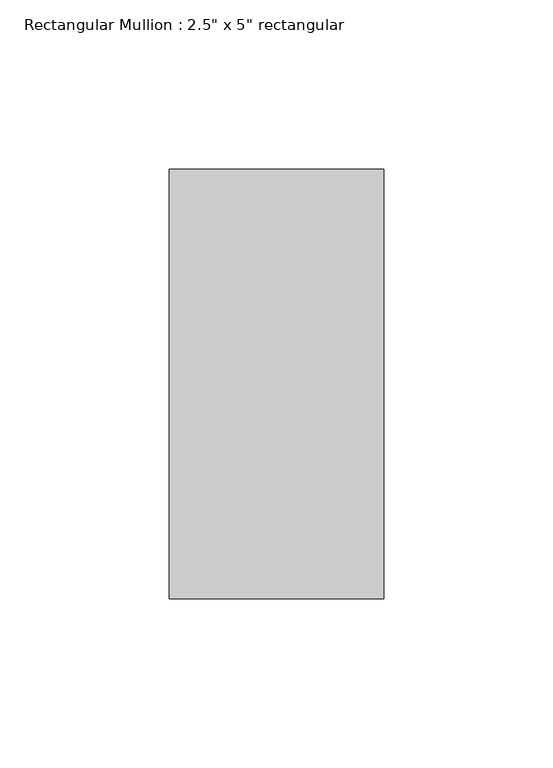
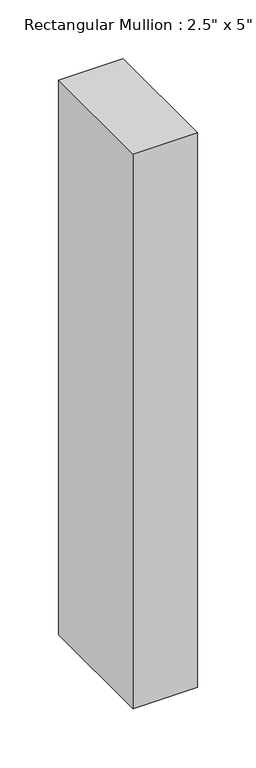
"""IFC4 building model written with IfcOpenShell, lengths in millimetres: member geometry."""

from ifc_helpers import new_model, si_unit, frame, origin, place, context, project, spatial, polyline, outline, extrude, source, transform, mapped, element, save


def member_af2dc76d(model_context):
    return source(origin(), model_context, "Body", "SweptSolid", [
        extrude(outline(polyline([(0.0, 63.5), (0.0, -63.5), (-63.5, -63.5), (-63.5, 63.5), (0.0, 63.5)])), frame((0.0, 0.0, -577.9826807), z_axis=(0.0, 0.0, 1.0), x_axis=(1.0, 0.0, 0.0)), (0.0, 0.0, 1.0), 577.9826807),
    ])


if __name__ == "__main__":
    model = new_model("IFC4")
    model_context = context("Model", 3, world=origin())
    ifc_project = project(units=[si_unit("LENGTHUNIT", "METRE", prefix="MILLI")], contexts=[model_context])
    site = spatial("IfcSite", under=ifc_project)
    building = spatial("IfcBuilding", under=site)
    placement = place(None, origin())
    member_shape = member_af2dc76d(model_context)
    element("IfcMember", 1, ObjectType="Rectangular Mullion : 2.5\" x 5\" rectangular", at=placement, inside=building, context=model_context, shape_type="MappedRepresentation", body=[
        mapped(member_shape, transform((0.0, 0.0, 0.0), x_axis=(1.0, 0.0, 0.0), y_axis=(0.0, 1.0, 0.0), z_axis=(0.0, 0.0, 1.0))),
    ])
    save(model, "model.ifc")

# Revit data of these elements
# Type "Rectangular Mullion : 2.5\" x 5\" rectangular"
#   built-in parameter 1007304 = 0.416667 (stored number, unit not read)
#   built-in parameter 1007301 = 0.104167 (stored number, unit not read)
#   built-in parameter 1007300 = 0.104167 (stored number, unit not read)
# Element 1 (IfcMember, "Rectangular Mullion : 2.5\" x 5\" rectangular")
#   Materials on its faces: "Aluminum"
# Materials
#   "Aluminum": class "Metal", colour RGB 247 247 247, transparency 0, Description = "Aluminum 6061", Cost = 0
